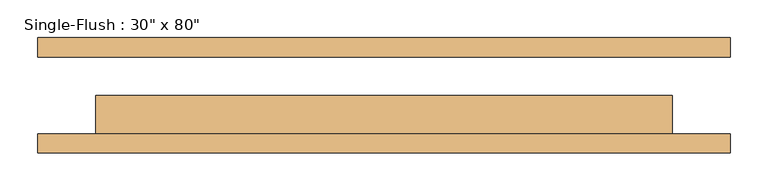
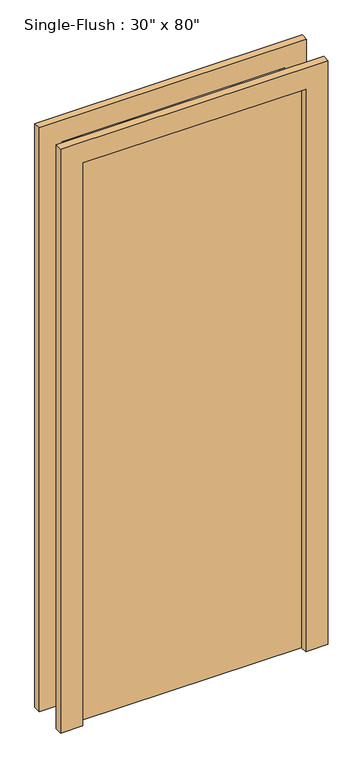
"""IFC4 building model written with IfcOpenShell, lengths in millimetres: door geometry."""

from ifc_helpers import new_model, si_unit, frame, origin, origin_with_axes, place, context, project, spatial, polyline, outline, extrude, source, transform, mapped, element, save


def door_98b18196(model_context):
    return source(origin(), model_context, "Body", "SweptSolid", [
        extrude(outline(polyline([(2108.2, -457.2), (0.0, -457.2), (0.0, -381.0), (2032.0, -381.0), (2032.0, 381.0), (0.0, 381.0), (0.0, 457.2), (2108.2, 457.2), (2108.2, -457.2)])), frame((0.0, -76.2, 0.0), z_axis=(0.0, 1.0, 0.0), x_axis=(0.0, 0.0, 1.0)), (0.0, 0.0, 1.0), 25.4),
        extrude(outline(polyline([(2108.2, 457.2), (2108.2, -457.2), (0.0, -457.2), (0.0, -381.0), (2032.0, -381.0), (2032.0, 381.0), (0.0, 381.0), (0.0, 457.2), (2108.2, 457.2)])), frame((0.0, 50.8, 0.0), z_axis=(0.0, 1.0, 0.0), x_axis=(0.0, 0.0, 1.0)), (0.0, 0.0, 1.0), 25.4),
        extrude(outline(polyline([(381.0, 0.0), (381.0, -50.8), (-381.0, -50.8), (-381.0, 0.0), (381.0, 0.0)])), origin_with_axes(), (0.0, 0.0, 1.0), 2032.0),
    ])


if __name__ == "__main__":
    model = new_model("IFC4")
    model_context = context("Model", 3, world=origin())
    ifc_project = project(units=[si_unit("LENGTHUNIT", "METRE", prefix="MILLI")], contexts=[model_context])
    site = spatial("IfcSite", under=ifc_project)
    building = spatial("IfcBuilding", under=site)
    placement = place(None, origin())
    door_shape = door_98b18196(model_context)
    element("IfcDoor", 1, ObjectType="Single-Flush : 30\" x 80\"", at=placement, inside=building, context=model_context, shape_type="MappedRepresentation", body=[
        mapped(door_shape, transform((0.0, 0.0, 0.0), x_axis=(1.0, 0.0, 0.0), y_axis=(0.0, 1.0, 0.0), z_axis=(0.0, 0.0, 1.0))),
    ])
    save(model, "model.ifc")

# Revit data of these elements
# Type "Single-Flush : 30\" x 80\""
#   Type Mark = "5"
#   Construction Type Id = "MDOOR"
#   Assembly Code = "C1020"
#   Analytic Construction = "Metal"
#   Thickness = 0' - 2"
#   Heat Transfer Coefficient (U) = 0.651978 BTU/(h·ft²·°F)
#   Height = 6' - 8"
#   Trim Projection Ext = 0' - 1"
#   Trim Projection Int = 0' - 1"
#   Trim Width = 0' - 3"
#   Width = 2' - 6"
#   Define Thermal Properties by = 1
#   Door Material = Door - Panel
#   Frame Material = Door - Frame
#   Visual Light Transmittance = 0
#   Solar Heat Gain Coefficient = 0
#   Function = (empty or 0)
#   Wall Closure = (empty or 0)
# Element 1 (IfcDoor, "Single-Flush : 30\" x 80\"")
#   Materials on its faces: "Door - Frame", "Door - Panel"
# Materials
#   "Door - Panel": class "Wood", colour RGB 210 159 95, transparency 0
#   "Door - Frame": colour RGB 118 70 51, transparency 0
